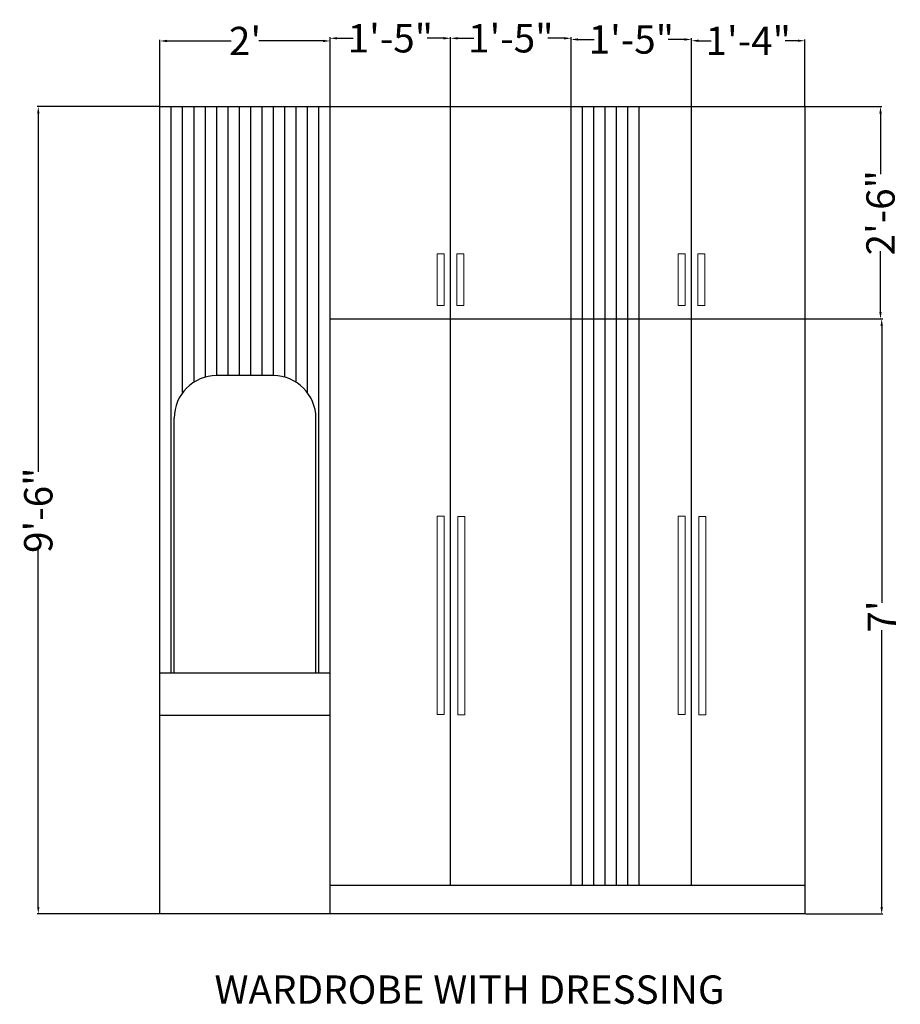
# Model space of a CAD drawing. Units: inches. Extents: x 231 to 355, y 183 to 322.
import ezdxf

# ---------------------------------------------------------------- set-up
doc = ezdxf.new("R2010")
doc.units = ezdxf.units.IN
doc.header["$MEASUREMENT"] = 0
for name, color, linetype, lineweight in [('A-ANNO-DIMS', 2, 'Continuous', 18), ('A-ANNO-TEXT', 7, 'Continuous', 25), ('A-FURN', 7, 'Continuous', 25), ('A-FURN-HDWR', 8, 'Continuous', 18)]:
    doc.layers.add(name, color=color, linetype=linetype, lineweight=lineweight)
doc.styles.get("Standard").update_dxf_attribs({"font": 'arial.ttf'})
doc.dimstyles.get("Standard").update_dxf_attribs({"dimtxt": 4, "dimasz": 1, "dimexe": 0.18, "dimexo": 0.0625, "dimgap": 0.09, "dimtad": 0, "dimdec": 0, "dimzin": 0, "dimdsep": 46, "dimlunit": 4, "dimtxsty": 'Standard', "dimcen": 0.09, "dimadec": 0, "dimazin": 0, "dimtfac": 1, "dimtdec": 0, "dimtofl": 0, "dimtmove": 0, "dimatfit": 3, "dimfxl": 1, "dimtolj": 1, "dimtzin": 0, "dimarcsym": 1})

# ---------------------------------------------------------------- blocks, each defined once
blk = doc.blocks.new('*D1')
at = {"layer": 'A-ANNO-DIMS', "color": 0, "lineweight": -2, "transparency": 16777216}
for p, q in [((325.57, 310.1), (325.57, 319.5)), ((326.57, 319.32), (328.35, 319.32)), ((340.57, 319.32), (338.79, 319.32)), ((341.57, 310.1), (341.57, 319.5))]:
    blk.add_line(p, q, dxfattribs=at)
at = {"layer": 'A-ANNO-DIMS', "color": 0, "transparency": 16777216}
for points in [[(326.57, 319.49), (326.57, 319.16), (325.57, 319.32)], [(340.57, 319.49), (340.57, 319.16), (341.57, 319.32)]]:
    blk.add_solid(points, dxfattribs=at)
at = {"layer": 'Defpoints', "color": 0, "transparency": 16777216}
for p in [(341.57, 319.32), (325.57, 310.04), (341.57, 310.04)]:
    blk.add_point(p, dxfattribs=at)
at = {"layer": 'A-ANNO-DIMS', "color": 0, "transparency": 16777216, "insert": (333.57, 319.32), "char_height": 4, "attachment_point": 5}
blk.add_mtext('\\A1;1\'-4"', dxfattribs=at)
blk = doc.blocks.new('*D2')
at = {"layer": 'A-ANNO-DIMS', "color": 0, "lineweight": -2, "transparency": 16777216}
for p, q in [((308.57, 310.1), (308.57, 319.68)), ((309.57, 319.5), (311.85, 319.5)), ((324.57, 319.5), (322.29, 319.5)), ((325.57, 310.1), (325.57, 319.68))]:
    blk.add_line(p, q, dxfattribs=at)
at = {"layer": 'A-ANNO-DIMS', "color": 0, "transparency": 16777216}
for points in [[(309.57, 319.67), (309.57, 319.34), (308.57, 319.5)], [(324.57, 319.67), (324.57, 319.34), (325.57, 319.5)]]:
    blk.add_solid(points, dxfattribs=at)
at = {"layer": 'Defpoints', "color": 0, "transparency": 16777216}
for p in [(325.57, 319.5), (308.57, 310.04), (325.57, 310.04)]:
    blk.add_point(p, dxfattribs=at)
at = {"layer": 'A-ANNO-DIMS', "color": 0, "transparency": 16777216, "insert": (317.07, 319.5), "char_height": 4, "attachment_point": 5}
blk.add_mtext('\\A1;1\'-5"', dxfattribs=at)
blk = doc.blocks.new('*D3')
at = {"layer": 'A-ANNO-DIMS', "color": 0, "lineweight": -2, "transparency": 16777216}
for p, q in [((291.57, 310.1), (291.57, 319.85)), ((308.57, 310.1), (308.57, 319.85)), ((292.57, 319.67), (294.85, 319.67)), ((307.57, 319.67), (305.29, 319.67))]:
    blk.add_line(p, q, dxfattribs=at)
at = {"layer": 'A-ANNO-DIMS', "color": 0, "transparency": 16777216}
for points in [[(292.57, 319.84), (292.57, 319.5), (291.57, 319.67)], [(307.57, 319.84), (307.57, 319.5), (308.57, 319.67)]]:
    blk.add_solid(points, dxfattribs=at)
at = {"layer": 'Defpoints', "color": 0, "transparency": 16777216}
for p in [(308.57, 319.67), (291.57, 310.04), (308.57, 310.04)]:
    blk.add_point(p, dxfattribs=at)
at = {"layer": 'A-ANNO-DIMS', "color": 0, "transparency": 16777216, "insert": (300.07, 319.67), "char_height": 4, "attachment_point": 5}
blk.add_mtext('\\A1;1\'-5"', dxfattribs=at)
blk = doc.blocks.new('*D4')
at = {"layer": 'A-ANNO-DIMS', "color": 0, "lineweight": -2, "transparency": 16777216}
for p, q in [((274.57, 310.1), (274.57, 319.85)), ((291.57, 310.1), (291.57, 319.85)), ((275.57, 319.67), (277.85, 319.67)), ((290.57, 319.67), (288.29, 319.67))]:
    blk.add_line(p, q, dxfattribs=at)
at = {"layer": 'A-ANNO-DIMS', "color": 0, "transparency": 16777216}
for points in [[(275.57, 319.84), (275.57, 319.5), (274.57, 319.67)], [(290.57, 319.84), (290.57, 319.5), (291.57, 319.67)]]:
    blk.add_solid(points, dxfattribs=at)
at = {"layer": 'Defpoints', "color": 0, "transparency": 16777216}
for p in [(291.57, 319.67), (274.57, 310.04), (291.57, 310.04)]:
    blk.add_point(p, dxfattribs=at)
at = {"layer": 'A-ANNO-DIMS', "color": 0, "transparency": 16777216, "insert": (283.07, 319.67), "char_height": 4, "attachment_point": 5}
blk.add_mtext('\\A1;1\'-5"', dxfattribs=at)
blk = doc.blocks.new('*D5')
at = {"layer": 'A-ANNO-DIMS', "color": 0, "lineweight": -2, "transparency": 16777216}
for p, q in [((250.57, 310.1), (250.57, 319.47)), ((251.57, 319.29), (260.61, 319.29)), ((273.57, 319.29), (264.54, 319.29)), ((274.57, 310.1), (274.57, 319.47))]:
    blk.add_line(p, q, dxfattribs=at)
at = {"layer": 'A-ANNO-DIMS', "color": 0, "transparency": 16777216}
for points in [[(251.57, 319.46), (251.57, 319.12), (250.57, 319.29)], [(273.57, 319.46), (273.57, 319.12), (274.57, 319.29)]]:
    blk.add_solid(points, dxfattribs=at)
at = {"layer": 'Defpoints', "color": 0, "transparency": 16777216}
for p in [(250.57, 319.29), (250.57, 310.04), (274.57, 310.04)]:
    blk.add_point(p, dxfattribs=at)
at = {"layer": 'A-ANNO-DIMS', "color": 0, "transparency": 16777216, "insert": (262.57, 319.29), "char_height": 4, "attachment_point": 5}
blk.add_mtext("\\A1;2'", dxfattribs=at)
blk = doc.blocks.new('*D6')
at = {"layer": 'A-ANNO-DIMS', "color": 0, "lineweight": -2, "transparency": 16777216}
for p, q in [((250.51, 310.04), (233.22, 310.04)), ((233.4, 309.04), (233.4, 258.44)), ((233.4, 197.04), (233.4, 247.63)), ((250.51, 196.04), (233.22, 196.04))]:
    blk.add_line(p, q, dxfattribs=at)
at = {"layer": 'A-ANNO-DIMS', "color": 0, "transparency": 16777216}
for points in [[(233.24, 309.04), (233.57, 309.04), (233.4, 310.04)], [(233.24, 197.04), (233.57, 197.04), (233.4, 196.04)]]:
    blk.add_solid(points, dxfattribs=at)
at = {"layer": 'Defpoints', "color": 0, "transparency": 16777216}
for p in [(233.4, 310.04), (250.57, 310.04), (250.57, 196.04)]:
    blk.add_point(p, dxfattribs=at)
at = {"layer": 'A-ANNO-DIMS', "color": 0, "transparency": 16777216, "insert": (233.4, 253.04), "char_height": 4, "attachment_point": 5, "rotation": 90}
blk.add_mtext('\\A1;9\'-6"', dxfattribs=at)
blk = doc.blocks.new('*D7')
at = {"layer": 'A-ANNO-DIMS', "color": 0, "lineweight": -2, "transparency": 16777216}
for p, q in [((341.63, 310.04), (352.41, 310.04)), ((352.23, 309.04), (352.23, 300.48)), ((352.23, 281.04), (352.23, 289.6)), ((341.63, 280.04), (352.41, 280.04))]:
    blk.add_line(p, q, dxfattribs=at)
at = {"layer": 'A-ANNO-DIMS', "color": 0, "transparency": 16777216}
for points in [[(352.07, 309.04), (352.4, 309.04), (352.23, 310.04)], [(352.07, 281.04), (352.4, 281.04), (352.23, 280.04)]]:
    blk.add_solid(points, dxfattribs=at)
at = {"layer": 'Defpoints', "color": 0, "transparency": 16777216}
for p in [(341.57, 310.04), (352.23, 310.04), (341.57, 280.04)]:
    blk.add_point(p, dxfattribs=at)
at = {"layer": 'A-ANNO-DIMS', "color": 0, "transparency": 16777216, "insert": (352.23, 295.04), "char_height": 4, "attachment_point": 5, "rotation": 90}
blk.add_mtext('\\A1;2\'-6"', dxfattribs=at)
blk = doc.blocks.new('*D8')
at = {"layer": 'A-ANNO-DIMS', "color": 0, "lineweight": -2, "transparency": 16777216}
for p, q in [((341.63, 280.04), (352.58, 280.04)), ((352.4, 279.04), (352.4, 239.95)), ((352.4, 197.04), (352.4, 236.12)), ((341.63, 196.04), (352.58, 196.04))]:
    blk.add_line(p, q, dxfattribs=at)
at = {"layer": 'A-ANNO-DIMS', "color": 0, "transparency": 16777216}
for points in [[(352.23, 279.04), (352.57, 279.04), (352.4, 280.04)], [(352.23, 197.04), (352.57, 197.04), (352.4, 196.04)]]:
    blk.add_solid(points, dxfattribs=at)
at = {"layer": 'Defpoints', "color": 0, "transparency": 16777216}
for p in [(341.57, 280.04), (341.57, 196.04), (352.4, 196.04)]:
    blk.add_point(p, dxfattribs=at)
at = {"layer": 'A-ANNO-DIMS', "color": 0, "transparency": 16777216, "insert": (352.4, 238.04), "char_height": 4, "attachment_point": 5, "rotation": 90}
blk.add_mtext("\\A1;7'", dxfattribs=at)
blk = doc.blocks.new('HANDLE-LOFT')
blk.add_line((0, 0), (1, 0))
blk.add_lwpolyline([(1, 0), (1, 7.29), (0, 7.29), (0, 0)])
blk = doc.blocks.new('HANDLE-SHUTTER-700')
blk.add_lwpolyline([(0, 0), (1, 0), (1, 28), (0, 28)], close=True)

msp = doc.modelspace()

# ---------------------------------------------------------------- linework, layer by layer
at = {"layer": 'A-FURN'}
for p, q in [((250.57, 310.04), (341.57, 310.04)), ((250.57, 196.04), (250.57, 310.04)), ((252.17, 230.04), (252.17, 310.04)), ((253.77, 269.64), (253.77, 310.04)), ((255.37, 271.11), (255.37, 310.04)), ((256.97, 271.82), (256.97, 310.04)), ((258.57, 272.04), (258.57, 310.04)), ((260.17, 272.04), (260.17, 310.04)), ((261.77, 272.04), (261.77, 310.04)), ((263.37, 272.04), (263.37, 310.04)), ((264.97, 272.04), (264.97, 310.04)), ((266.57, 272.04), (266.57, 310.04)), ((268.17, 271.82), (268.17, 310.04)), ((269.77, 271.11), (269.77, 310.04)), ((271.37, 269.64), (271.37, 310.04)), ((272.97, 230.04), (272.97, 310.04)), ((274.57, 196.04), (274.57, 310.04)), ((291.57, 200.04), (291.57, 310.04)), ((308.57, 200.04), (308.57, 310.04)), ((310.17, 200.04), (310.17, 310.04)), ((311.77, 200.04), (311.77, 310.04)), ((313.37, 200.04), (313.37, 310.04)), ((314.97, 200.04), (314.97, 310.04)), ((316.57, 200.04), (316.57, 310.04)), ((318.17, 200.04), (318.17, 310.04)), ((325.57, 200.04), (325.57, 310.04)), ((341.57, 310.04), (341.57, 196.04)), ((274.57, 280.04), (341.57, 280.04)), ((266.57, 272.04), (258.57, 272.04)), ((252.57, 230.04), (252.57, 266.04)), ((272.57, 230.04), (272.57, 266.04)), ((274.57, 230.04), (250.57, 230.04)), ((274.57, 224.04), (250.57, 224.04)), ((341.57, 200.04), (274.57, 200.04)), ((341.57, 196.04), (250.57, 196.04))]:
    msp.add_line(p, q, dxfattribs=at)
for centre, start, end in [((258.57, 266.04), 90, 180), ((266.57, 266.04), 0, 90)]:
    msp.add_arc(centre, 6, start, end, dxfattribs=at)

# ---------------------------------------------------------------- block references
at = {"layer": 'A-FURN-HDWR'}
for name, p in [('HANDLE-LOFT', (289.68, 281.95)), ('HANDLE-LOFT', (292.46, 281.95)), ('HANDLE-LOFT', (323.68, 281.95)), ('HANDLE-LOFT', (326.46, 281.95)), ('HANDLE-SHUTTER-700', (289.69, 224.19)), ('HANDLE-SHUTTER-700', (292.58, 224.16)), ('HANDLE-SHUTTER-700', (323.69, 224.19)), ('HANDLE-SHUTTER-700', (326.58, 224.16))]:
    msp.add_blockref(name, p, dxfattribs=at)

# ---------------------------------------------------------------- texts
at = {"layer": 'A-ANNO-TEXT', "insert": (252.21, 187.36), "char_height": 4, "attachment_point": 1}
msp.add_mtext_dynamic_manual_height_columns('\\pxqc;WARDROBE WITH DRESSING', width=84.0756, gutter_width=20, heights=[0], dxfattribs=at)

# ---------------------------------------------------------------- dimensions: what is measured, and where the dimension line sits
at = {"layer": 'A-ANNO-DIMS'}
for base, p1, p2, picture, middle in [((250.57, 319.29), (274.57, 310.04), (250.57, 310.04), '*D5', (262.57, 319.29)), ((291.57, 319.67), (274.57, 310.04), (291.57, 310.04), '*D4', (283.07, 319.67)), ((308.57, 319.67), (291.57, 310.04), (308.57, 310.04), '*D3', (300.07, 319.67)), ((325.57, 319.5), (308.57, 310.04), (325.57, 310.04), '*D2', (317.07, 319.5)), ((341.57, 319.32), (325.57, 310.04), (341.57, 310.04), '*D1', (333.57, 319.32))]:
    dim = msp.add_linear_dim(base=base, p1=p1, p2=p2, dimstyle='Standard', override={"dimclrd": 0, "dimclre": 0, "dimclrt": 0}, dxfattribs=at)
    dim.commit()
    dim.dimension.update_dxf_attribs({"geometry": picture, "text_midpoint": middle})
for base, p1, p2, picture, middle in [((233.4, 310.04), (250.57, 196.04), (250.57, 310.04), '*D6', (233.4, 253.04)), ((352.23, 310.04), (341.57, 280.04), (341.57, 310.04), '*D7', (352.23, 295.04)), ((352.4, 196.04), (341.57, 280.04), (341.57, 196.04), '*D8', (352.4, 238.04))]:
    dim = msp.add_linear_dim(base=base, p1=p1, p2=p2, angle=90, dimstyle='Standard', override={"dimclrd": 0, "dimclre": 0, "dimclrt": 0}, dxfattribs=at)
    dim.commit()
    dim.dimension.update_dxf_attribs({"geometry": picture, "text_midpoint": middle})

doc.saveas('drawing.dxf')
